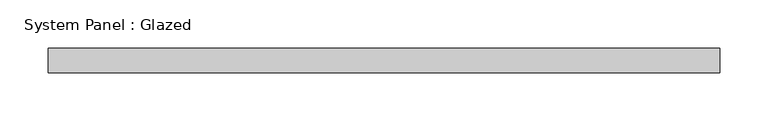
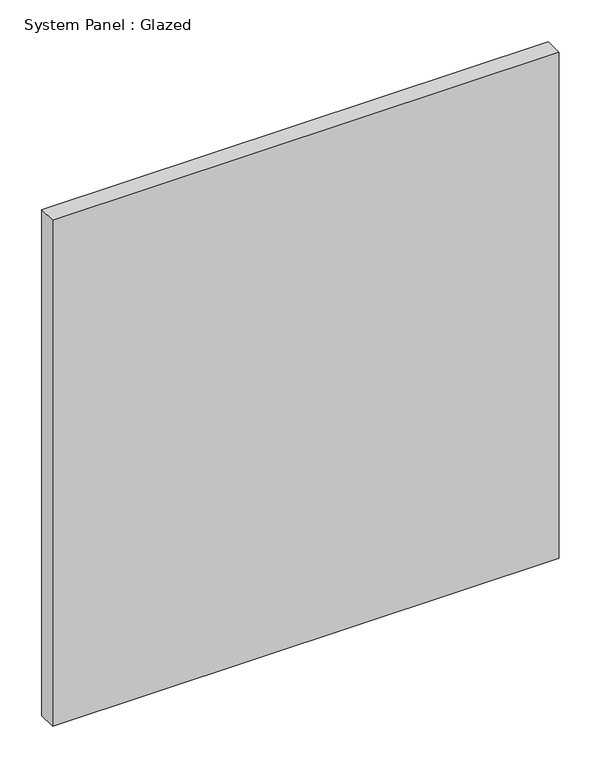
"""IFC4 building model written with IfcOpenShell, lengths in millimetres: plate geometry, System Panel : Glazed."""

from ifc_helpers import new_model, si_unit, origin, origin_with_axes, place, context, project, spatial, polyline, outline, extrude, source, transform, mapped, element, save


def system_panel_glazed_b47efb59(model_context):
    return source(origin(), model_context, "Body", "SweptSolid", [
        extrude(outline(polyline([(349.25, 19.05), (-349.25, 19.05), (-349.25, 44.45), (349.25, 44.45), (349.25, 19.05)])), origin_with_axes(), (0.0, 0.0, 1.0), 737.2861093),
    ])


if __name__ == "__main__":
    model = new_model("IFC4")
    model_context = context("Model", 3, world=origin())
    ifc_project = project(units=[si_unit("LENGTHUNIT", "METRE", prefix="MILLI")], contexts=[model_context])
    site = spatial("IfcSite", under=ifc_project)
    building = spatial("IfcBuilding", under=site)
    placement = place(None, origin())
    system_panel_glazed_shape = system_panel_glazed_b47efb59(model_context)
    element("IfcPlate", 1, ObjectType="System Panel : Glazed", at=placement, inside=building, context=model_context, shape_type="MappedRepresentation", body=[
        mapped(system_panel_glazed_shape, transform((0.0, 0.0, 0.0), x_axis=(1.0, 0.0, 0.0), y_axis=(0.0, 1.0, 0.0), z_axis=(0.0, 0.0, 1.0))),
    ])
    save(model, "model.ifc")

# Revit data of these elements
# Type "System Panel : Glazed"
#   Construction Type Id = "GSP4R"
#   Analytic Construction = "1/8 in Pilkington single glazing"
#   Visual Light Transmittance = 0.9
#   Solar Heat Gain Coefficient = 0.86
#   Heat Transfer Coefficient (U) = 1.18115 BTU/(h·ft²·°F)
#   Define Thermal Properties by = 1
# Element 1 (IfcPlate, "System Panel : Glazed")
#   Materials on its faces: "Glass"
# Materials
#   "Glass": class "Glass", colour RGB 0 128 192, transparency 0.75, Description = "Soda Lime Glass", Cost = 0
